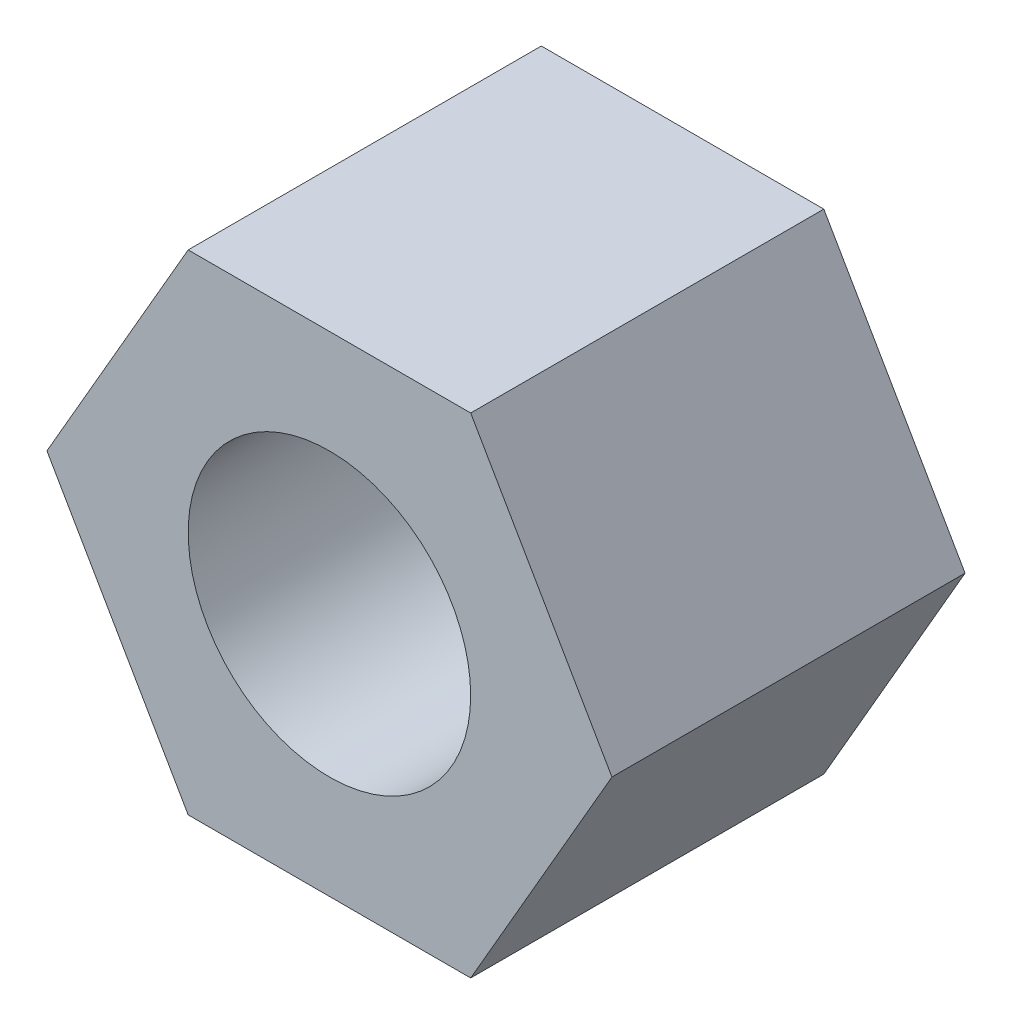
SolidWorks part; units mm, degrees
material "Plain Carbon Steel"
ref_plane "Front Plane" through (0, 0, 0) normal (0, 0, 1) x (1, 0, 0)
ref_plane "Top Plane" through (0, 0, 0) normal (0, 1, 0) x (1, 0, 0)
ref_plane "Right Plane" through (0, 0, 0) normal (1, 0, 0) x (0, 0, -1)
sketch "Hex Profile with Bore Ø12" plane through (0, 0, 0) normal (0, 0, 1) x (1, 0, 0)
  line L1 (12, 0) -> (6, 10.3923)
  line L2 (6, 10.3923) -> (-6, 10.3923)
  line L3 (-6, 10.3923) -> (-12, 0)
  line L4 (-12, 0) -> (-6, -10.3923)
  line L5 (-6, -10.3923) -> (6, -10.3923)
  line L6 (6, -10.3923) -> (12, 0)
  circle A0 centre (0, 0) radius 12 construction
  circle A1 centre (0, 0) radius 6
  dimension "D1" = 24
  dimension "D2" = 12
extrude "Hex Body 15mm" add sketch "Hex Profile with Bore Ø12" along normal blind 15
